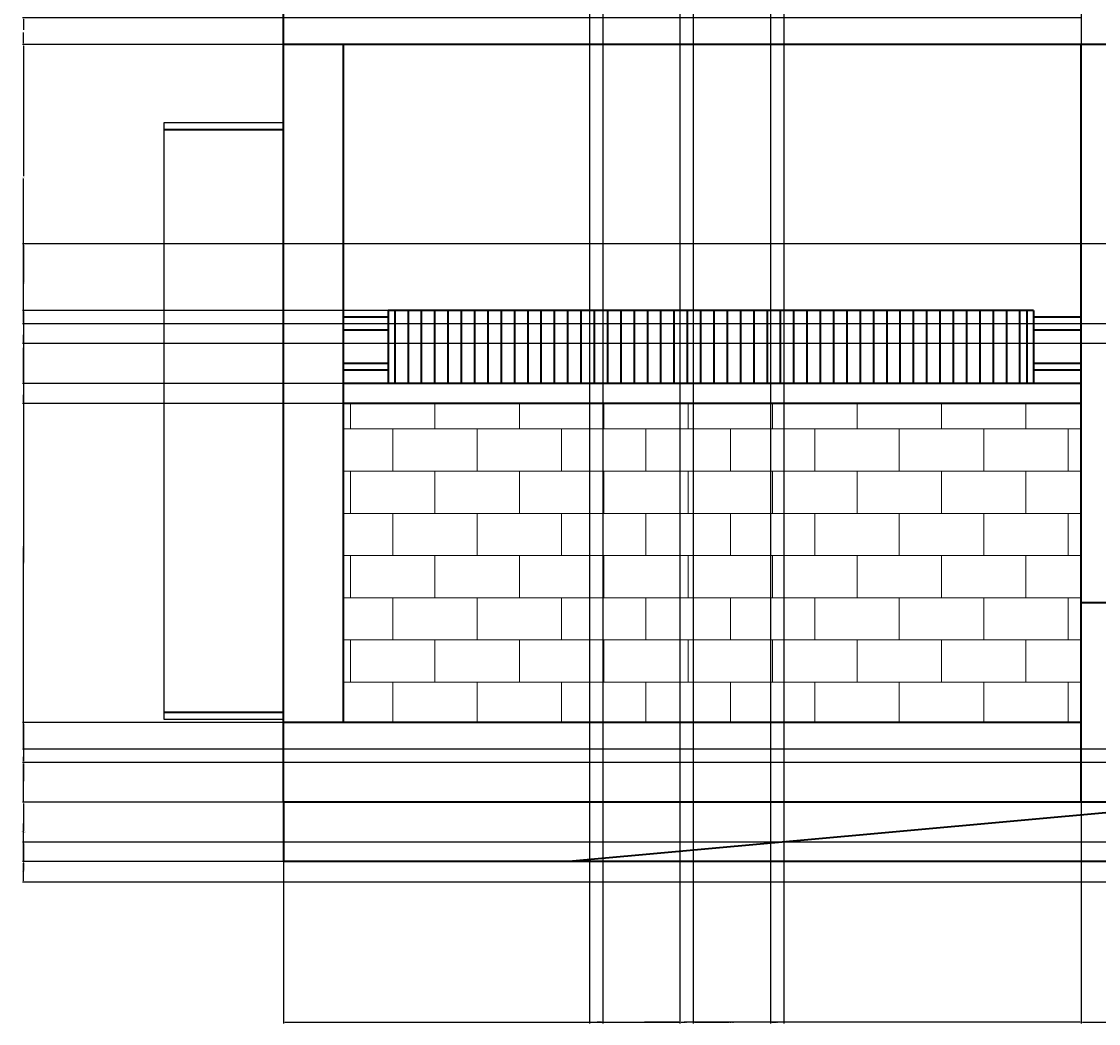
# Model space of a CAD drawing. Units: inches. Extents: x 2148 to 2587, y 1015 to 1466.
# Tile 1 of 7: x 2148 to 2310, y 1015 to 1166. Entities that reach past the tile are written whole.
import ezdxf

# ---------------------------------------------------------------- set-up
doc = ezdxf.new("R2010")
doc.units = ezdxf.units.IN
for name, color, linetype, lineweight in [('A-ANNO-DIMS', 2, 'Continuous', 18), ('A-ELEV', 7, 'Continuous', 35), ('A-GLAZ', 4, 'Continuous', 25), ('A-WALL-PATT', 8, 'Continuous', 18)]:
    doc.layers.add(name, color=color, linetype=linetype, lineweight=lineweight)
doc.styles.get("Standard").update_dxf_attribs({"font": 'arial.ttf'})
doc.dimstyles.get("Standard").update_dxf_attribs({"dimtxt": 0.18, "dimasz": 0.18, "dimexe": 0.18, "dimexo": 0.0625, "dimgap": 0.09, "dimtad": 0, "dimtih": 1, "dimtoh": 1, "dimdec": 4, "dimzin": 0, "dimdsep": 46, "dimtxsty": 'Standard', "dimcen": 0.09, "dimadec": 0, "dimazin": 0, "dimtfac": 1, "dimtdec": 4, "dimtofl": 0, "dimtmove": 0, "dimatfit": 3, "dimfxl": 1, "dimtolj": 1, "dimtzin": 0, "dimarcsym": 0})

# ---------------------------------------------------------------- blocks, each defined once
blk = doc.blocks.new('WIN-SIDE')
for p, q in [((18, 89.73), (0, 89.73)), ((18, 0), (18, 89.73)), ((0, 0), (18, 0))]:
    blk.add_line(p, q)
blk = doc.blocks.new('*D10')
at = {"layer": 'A-ANNO-DIMS', "color": 0, "lineweight": -2, "transparency": 16777216}
for p, q in [((2307.03, 1048.68), (2307.03, 1015.46)), ((2187.03, 1039.75), (2187.03, 1015.46)), ((2187.21, 1015.64), (2246.75, 1015.64)), ((2306.85, 1015.64), (2247.31, 1015.64))]:
    blk.add_line(p, q, dxfattribs=at)
at = {"layer": 'A-ANNO-DIMS', "color": 0, "transparency": 16777216}
for points in [[(2187.21, 1015.67), (2187.21, 1015.61), (2187.03, 1015.64)], [(2306.85, 1015.67), (2306.85, 1015.61), (2307.03, 1015.64)]]:
    blk.add_solid(points, dxfattribs=at)
at = {"layer": 'Defpoints', "color": 0, "transparency": 16777216}
for p in [(2307.03, 1048.74), (2187.03, 1039.82), (2307.03, 1015.64)]:
    blk.add_point(p, dxfattribs=at)
at = {"layer": 'A-ANNO-DIMS', "color": 0, "transparency": 16777216, "insert": (2247.03, 1015.64), "char_height": 0.18, "attachment_point": 5}
blk.add_mtext('\\A1;120', dxfattribs=at)
blk = doc.blocks.new('*D11')
at = {"layer": 'A-ANNO-DIMS', "color": 0, "lineweight": -2, "transparency": 16777216}
for p, q in [((2307.03, 1048.68), (2307.03, 1015.46)), ((2316.03, 1048.68), (2316.03, 1015.46)), ((2307.21, 1015.64), (2311.39, 1015.64)), ((2315.85, 1015.64), (2311.68, 1015.64))]:
    blk.add_line(p, q, dxfattribs=at)
at = {"layer": 'A-ANNO-DIMS', "color": 0, "transparency": 16777216}
for points in [[(2307.21, 1015.67), (2307.21, 1015.61), (2307.03, 1015.64)], [(2315.85, 1015.67), (2315.85, 1015.61), (2316.03, 1015.64)]]:
    blk.add_solid(points, dxfattribs=at)
at = {"layer": 'Defpoints', "color": 0, "transparency": 16777216}
for p in [(2307.03, 1048.74), (2316.03, 1048.74), (2316.03, 1015.64)]:
    blk.add_point(p, dxfattribs=at)
at = {"layer": 'A-ANNO-DIMS', "color": 0, "transparency": 16777216, "insert": (2311.53, 1015.64), "char_height": 0.18, "attachment_point": 5}
blk.add_mtext('\\A1;9', dxfattribs=at)
blk = doc.blocks.new('*D16')
at = {"layer": 'A-ANNO-DIMS', "color": 0, "lineweight": -2, "transparency": 16777216}
for p, q in [((2186.97, 1048.74), (2147.75, 1048.74)), ((2147.93, 1048.56), (2147.93, 1044.46)), ((2147.93, 1040), (2147.93, 1044.1)), ((2186.97, 1039.82), (2147.75, 1039.82))]:
    blk.add_line(p, q, dxfattribs=at)
at = {"layer": 'A-ANNO-DIMS', "color": 0, "transparency": 16777216}
for points in [[(2147.9, 1048.56), (2147.96, 1048.56), (2147.93, 1048.74)], [(2147.9, 1040), (2147.96, 1040), (2147.93, 1039.82)]]:
    blk.add_solid(points, dxfattribs=at)
at = {"layer": 'Defpoints', "color": 0, "transparency": 16777216}
for p in [(2147.93, 1048.74), (2187.03, 1048.74), (2187.03, 1039.82)]:
    blk.add_point(p, dxfattribs=at)
at = {"layer": 'A-ANNO-DIMS', "color": 0, "transparency": 16777216, "insert": (2147.93, 1044.28), "char_height": 0.18, "attachment_point": 5}
blk.add_mtext('\\A1;8.925', dxfattribs=at)
blk = doc.blocks.new('*D17')
at = {"layer": 'A-ANNO-DIMS', "color": 0, "lineweight": -2, "transparency": 16777216}
for p, q in [((2186.97, 1060.74), (2147.75, 1060.74)), ((2147.93, 1060.56), (2147.93, 1054.92)), ((2147.93, 1048.92), (2147.93, 1054.56)), ((2186.97, 1048.74), (2147.75, 1048.74))]:
    blk.add_line(p, q, dxfattribs=at)
at = {"layer": 'A-ANNO-DIMS', "color": 0, "transparency": 16777216}
for points in [[(2147.9, 1060.56), (2147.96, 1060.56), (2147.93, 1060.74)], [(2147.9, 1048.92), (2147.96, 1048.92), (2147.93, 1048.74)]]:
    blk.add_solid(points, dxfattribs=at)
at = {"layer": 'Defpoints', "color": 0, "transparency": 16777216}
for p in [(2147.93, 1060.74), (2187.03, 1060.74), (2187.03, 1048.74)]:
    blk.add_point(p, dxfattribs=at)
at = {"layer": 'A-ANNO-DIMS', "color": 0, "transparency": 16777216, "insert": (2147.93, 1054.74), "char_height": 0.18, "attachment_point": 5}
blk.add_mtext('\\A1;12', dxfattribs=at)
blk = doc.blocks.new('*D18')
at = {"layer": 'A-ANNO-DIMS', "color": 0, "lineweight": -2, "transparency": 16777216}
for p, q in [((2195.97, 1108.74), (2147.75, 1108.74)), ((2147.93, 1108.56), (2147.93, 1084.92)), ((2147.93, 1060.92), (2147.93, 1084.56)), ((2195.97, 1060.74), (2147.75, 1060.74))]:
    blk.add_line(p, q, dxfattribs=at)
at = {"layer": 'A-ANNO-DIMS', "color": 0, "transparency": 16777216}
for points in [[(2147.9, 1108.56), (2147.96, 1108.56), (2147.93, 1108.74)], [(2147.9, 1060.92), (2147.96, 1060.92), (2147.93, 1060.74)]]:
    blk.add_solid(points, dxfattribs=at)
at = {"layer": 'Defpoints', "color": 0, "transparency": 16777216}
for p in [(2147.93, 1108.74), (2196.03, 1108.74), (2196.03, 1060.74)]:
    blk.add_point(p, dxfattribs=at)
at = {"layer": 'A-ANNO-DIMS', "color": 0, "transparency": 16777216, "insert": (2147.93, 1084.74), "char_height": 0.18, "attachment_point": 5}
blk.add_mtext('\\A1;48', dxfattribs=at)
blk = doc.blocks.new('*D19')
at = {"layer": 'A-ANNO-DIMS', "color": 0, "lineweight": -2, "transparency": 16777216}
for p, q in [((2195.97, 1111.74), (2147.75, 1111.74)), ((2147.93, 1111.56), (2147.93, 1110.42)), ((2147.93, 1108.92), (2147.93, 1110.06)), ((2195.97, 1108.74), (2147.75, 1108.74))]:
    blk.add_line(p, q, dxfattribs=at)
at = {"layer": 'A-ANNO-DIMS', "color": 0, "transparency": 16777216}
for points in [[(2147.9, 1111.56), (2147.96, 1111.56), (2147.93, 1111.74)], [(2147.9, 1108.92), (2147.96, 1108.92), (2147.93, 1108.74)]]:
    blk.add_solid(points, dxfattribs=at)
at = {"layer": 'Defpoints', "color": 0, "transparency": 16777216}
for p in [(2147.93, 1111.74), (2196.03, 1111.74), (2196.03, 1108.74)]:
    blk.add_point(p, dxfattribs=at)
at = {"layer": 'A-ANNO-DIMS', "color": 0, "transparency": 16777216, "insert": (2147.93, 1110.24), "char_height": 0.18, "attachment_point": 5}
blk.add_mtext('\\A1;3', dxfattribs=at)
blk = doc.blocks.new('*D20')
at = {"layer": 'A-ANNO-DIMS', "color": 0, "lineweight": -2, "transparency": 16777216}
for p, q in [((2202.7, 1122.74), (2147.75, 1122.74)), ((2147.93, 1122.56), (2147.93, 1117.42)), ((2147.93, 1111.92), (2147.93, 1117.06)), ((2202.7, 1111.74), (2147.75, 1111.74))]:
    blk.add_line(p, q, dxfattribs=at)
at = {"layer": 'A-ANNO-DIMS', "color": 0, "transparency": 16777216}
for points in [[(2147.9, 1122.56), (2147.96, 1122.56), (2147.93, 1122.74)], [(2147.9, 1111.92), (2147.96, 1111.92), (2147.93, 1111.74)]]:
    blk.add_solid(points, dxfattribs=at)
at = {"layer": 'Defpoints', "color": 0, "transparency": 16777216}
for p in [(2147.93, 1122.74), (2202.76, 1122.74), (2202.76, 1111.74)]:
    blk.add_point(p, dxfattribs=at)
at = {"layer": 'A-ANNO-DIMS', "color": 0, "transparency": 16777216, "insert": (2147.93, 1117.24), "char_height": 0.18, "attachment_point": 5}
blk.add_mtext('\\A1;11', dxfattribs=at)
blk = doc.blocks.new('*D21')
at = {"layer": 'A-ANNO-DIMS', "color": 0, "lineweight": -2, "transparency": 16777216}
for p, q in [((2186.97, 1162.74), (2147.75, 1162.74)), ((2147.93, 1162.56), (2147.93, 1142.92)), ((2147.93, 1122.92), (2147.93, 1142.56)), ((2202.7, 1122.74), (2147.75, 1122.74))]:
    blk.add_line(p, q, dxfattribs=at)
at = {"layer": 'A-ANNO-DIMS', "color": 0, "transparency": 16777216}
for points in [[(2147.9, 1162.56), (2147.96, 1162.56), (2147.93, 1162.74)], [(2147.9, 1122.92), (2147.96, 1122.92), (2147.93, 1122.74)]]:
    blk.add_solid(points, dxfattribs=at)
at = {"layer": 'Defpoints', "color": 0, "transparency": 16777216}
for p in [(2147.93, 1162.74), (2187.03, 1162.74), (2202.76, 1122.74)]:
    blk.add_point(p, dxfattribs=at)
at = {"layer": 'A-ANNO-DIMS', "color": 0, "transparency": 16777216, "insert": (2147.93, 1142.74), "char_height": 0.18, "attachment_point": 5}
blk.add_mtext('\\A1;40', dxfattribs=at)
blk = doc.blocks.new('*D22')
at = {"layer": 'A-ANNO-DIMS', "color": 0, "lineweight": -2, "transparency": 16777216}
for p, q in [((2186.971769, 1166.74266), (2147.754269, 1166.74266)), ((2147.934269, 1166.56266), (2147.934269, 1164.92266)), ((2147.934269, 1162.92266), (2147.934269, 1164.56266)), ((2186.971769, 1162.74266), (2147.754269, 1162.74266))]:
    blk.add_line(p, q, dxfattribs=at)
at = {"layer": 'A-ANNO-DIMS', "color": 0, "transparency": 16777216}
for points in [[(2147.904269, 1166.56266), (2147.964269, 1166.56266), (2147.934269, 1166.74266)], [(2147.904269, 1162.92266), (2147.964269, 1162.92266), (2147.934269, 1162.74266)]]:
    blk.add_solid(points, dxfattribs=at)
at = {"layer": 'Defpoints', "color": 0, "transparency": 16777216}
for p in [(2147.934269, 1166.74266), (2187.034269, 1166.74266), (2187.034269, 1162.74266)]:
    blk.add_point(p, dxfattribs=at)
at = {"layer": 'A-ANNO-DIMS', "color": 0, "transparency": 16777216, "insert": (2147.934269, 1164.74266), "char_height": 0.18, "attachment_point": 5}
blk.add_mtext('\\A1;4', dxfattribs=at)
blk = doc.blocks.new('*D47')
at = {"layer": 'A-ANNO-DIMS', "color": 0, "lineweight": -2, "transparency": 16777216}
for p, q in [((2307.03, 1334.68), (2307.03, 1015.46)), ((2316.03, 1329.68), (2316.03, 1015.46)), ((2307.21, 1015.64), (2311.39, 1015.64)), ((2315.85, 1015.64), (2311.68, 1015.64))]:
    blk.add_line(p, q, dxfattribs=at)
at = {"layer": 'A-ANNO-DIMS', "color": 0, "transparency": 16777216}
for points in [[(2307.21, 1015.67), (2307.21, 1015.61), (2307.03, 1015.64)], [(2315.85, 1015.67), (2315.85, 1015.61), (2316.03, 1015.64)]]:
    blk.add_solid(points, dxfattribs=at)
at = {"layer": 'Defpoints', "color": 0, "transparency": 16777216}
for p in [(2307.03, 1334.74), (2316.03, 1329.74), (2316.03, 1015.64)]:
    blk.add_point(p, dxfattribs=at)
at = {"layer": 'A-ANNO-DIMS', "color": 0, "transparency": 16777216, "insert": (2311.53, 1015.64), "char_height": 0.18, "attachment_point": 5}
blk.add_mtext('\\A1;9', dxfattribs=at)
blk = doc.blocks.new('*D58')
at = {"layer": 'A-ANNO-DIMS', "color": 0, "lineweight": -2, "transparency": 16777216}
for p, q in [((2306.971769, 1166.74266), (2147.754269, 1166.74266)), ((2147.934269, 1166.56266), (2147.934269, 1164.92266)), ((2147.934269, 1162.92266), (2147.934269, 1164.56266)), ((2306.971769, 1162.74266), (2147.754269, 1162.74266))]:
    blk.add_line(p, q, dxfattribs=at)
at = {"layer": 'A-ANNO-DIMS', "color": 0, "transparency": 16777216}
for points in [[(2147.904269, 1166.56266), (2147.964269, 1166.56266), (2147.934269, 1166.74266)], [(2147.904269, 1162.92266), (2147.964269, 1162.92266), (2147.934269, 1162.74266)]]:
    blk.add_solid(points, dxfattribs=at)
at = {"layer": 'Defpoints', "color": 0, "transparency": 16777216}
for p in [(2147.934269, 1166.74266), (2307.034269, 1166.74266), (2307.034269, 1162.74266)]:
    blk.add_point(p, dxfattribs=at)
at = {"layer": 'A-ANNO-DIMS', "color": 0, "transparency": 16777216, "insert": (2147.934269, 1164.74266), "char_height": 0.18, "attachment_point": 5}
blk.add_mtext('\\A1;4', dxfattribs=at)
blk = doc.blocks.new('*D83')
at = {"layer": 'A-ANNO-DIMS', "color": 0, "lineweight": -2, "transparency": 16777216}
for p, q in [((2235.06, 1199.68), (2235.06, 1015.46)), ((2233.06, 1197.68), (2233.06, 1015.46)), ((2233.24, 1015.64), (2233.91, 1015.64)), ((2234.88, 1015.64), (2234.21, 1015.64))]:
    blk.add_line(p, q, dxfattribs=at)
at = {"layer": 'A-ANNO-DIMS', "color": 0, "transparency": 16777216}
for points in [[(2233.24, 1015.67), (2233.24, 1015.61), (2233.06, 1015.64)], [(2234.88, 1015.67), (2234.88, 1015.61), (2235.06, 1015.64)]]:
    blk.add_solid(points, dxfattribs=at)
at = {"layer": 'Defpoints', "color": 0, "transparency": 16777216}
for p in [(2235.06, 1199.74), (2233.06, 1197.74), (2235.06, 1015.64)]:
    blk.add_point(p, dxfattribs=at)
at = {"layer": 'A-ANNO-DIMS', "color": 0, "transparency": 16777216, "insert": (2234.06, 1015.64), "char_height": 0.18, "attachment_point": 5}
blk.add_mtext('\\A1;2', dxfattribs=at)
blk = doc.blocks.new('*D84')
at = {"layer": 'A-ANNO-DIMS', "color": 0, "lineweight": -2, "transparency": 16777216}
for p, q in [((2246.67, 1247.43), (2246.67, 1015.46)), ((2235.06, 1199.68), (2235.06, 1015.46)), ((2235.24, 1015.64), (2240.41, 1015.64)), ((2246.49, 1015.64), (2241.32, 1015.64))]:
    blk.add_line(p, q, dxfattribs=at)
at = {"layer": 'A-ANNO-DIMS', "color": 0, "transparency": 16777216}
for points in [[(2235.24, 1015.67), (2235.24, 1015.61), (2235.06, 1015.64)], [(2246.49, 1015.67), (2246.49, 1015.61), (2246.67, 1015.64)]]:
    blk.add_solid(points, dxfattribs=at)
at = {"layer": 'Defpoints', "color": 0, "transparency": 16777216}
for p in [(2246.67, 1247.49), (2235.06, 1199.74), (2246.67, 1015.64)]:
    blk.add_point(p, dxfattribs=at)
at = {"layer": 'A-ANNO-DIMS', "color": 0, "transparency": 16777216, "insert": (2240.87, 1015.64), "char_height": 0.18, "attachment_point": 5}
blk.add_mtext('\\A1;11.613', dxfattribs=at)
blk = doc.blocks.new('*D85')
at = {"layer": 'A-ANNO-DIMS', "color": 0, "lineweight": -2, "transparency": 16777216}
for p, q in [((2246.67, 1247.43), (2246.67, 1015.46)), ((2248.67, 1247.43), (2248.67, 1015.46)), ((2246.85, 1015.64), (2247.52, 1015.64)), ((2248.49, 1015.64), (2247.82, 1015.64))]:
    blk.add_line(p, q, dxfattribs=at)
at = {"layer": 'A-ANNO-DIMS', "color": 0, "transparency": 16777216}
for points in [[(2246.85, 1015.67), (2246.85, 1015.61), (2246.67, 1015.64)], [(2248.49, 1015.67), (2248.49, 1015.61), (2248.67, 1015.64)]]:
    blk.add_solid(points, dxfattribs=at)
at = {"layer": 'Defpoints', "color": 0, "transparency": 16777216}
for p in [(2246.67, 1247.49), (2248.67, 1247.49), (2248.67, 1015.64)]:
    blk.add_point(p, dxfattribs=at)
at = {"layer": 'A-ANNO-DIMS', "color": 0, "transparency": 16777216, "insert": (2247.67, 1015.64), "char_height": 0.18, "attachment_point": 5}
blk.add_mtext('\\A1;2', dxfattribs=at)
blk = doc.blocks.new('*D86')
at = {"layer": 'A-ANNO-DIMS', "color": 0, "lineweight": -2, "transparency": 16777216}
for p, q in [((2248.67, 1247.43), (2248.67, 1015.46)), ((2260.29, 1199.68), (2260.29, 1015.46)), ((2248.85, 1015.64), (2254.03, 1015.64)), ((2260.11, 1015.64), (2254.94, 1015.64))]:
    blk.add_line(p, q, dxfattribs=at)
at = {"layer": 'A-ANNO-DIMS', "color": 0, "transparency": 16777216}
for points in [[(2248.85, 1015.67), (2248.85, 1015.61), (2248.67, 1015.64)], [(2260.11, 1015.67), (2260.11, 1015.61), (2260.29, 1015.64)]]:
    blk.add_solid(points, dxfattribs=at)
at = {"layer": 'Defpoints', "color": 0, "transparency": 16777216}
for p in [(2248.67, 1247.49), (2260.29, 1199.74), (2260.29, 1015.64)]:
    blk.add_point(p, dxfattribs=at)
at = {"layer": 'A-ANNO-DIMS', "color": 0, "transparency": 16777216, "insert": (2254.48, 1015.64), "char_height": 0.18, "attachment_point": 5}
blk.add_mtext('\\A1;11.613', dxfattribs=at)
blk = doc.blocks.new('*D87')
at = {"layer": 'A-ANNO-DIMS', "color": 0, "lineweight": -2, "transparency": 16777216}
for p, q in [((2260.29, 1199.68), (2260.29, 1015.46)), ((2262.29, 1197.68), (2262.29, 1015.46)), ((2260.47, 1015.64), (2261.14, 1015.64)), ((2262.11, 1015.64), (2261.44, 1015.64))]:
    blk.add_line(p, q, dxfattribs=at)
at = {"layer": 'A-ANNO-DIMS', "color": 0, "transparency": 16777216}
for points in [[(2260.47, 1015.67), (2260.47, 1015.61), (2260.29, 1015.64)], [(2262.11, 1015.67), (2262.11, 1015.61), (2262.29, 1015.64)]]:
    blk.add_solid(points, dxfattribs=at)
at = {"layer": 'Defpoints', "color": 0, "transparency": 16777216}
for p in [(2260.29, 1199.74), (2262.29, 1197.74), (2262.29, 1015.64)]:
    blk.add_point(p, dxfattribs=at)
at = {"layer": 'A-ANNO-DIMS', "color": 0, "transparency": 16777216, "insert": (2261.29, 1015.64), "char_height": 0.18, "attachment_point": 5}
blk.add_mtext('\\A1;2', dxfattribs=at)
blk = doc.blocks.new('*D110')
at = {"layer": 'A-ANNO-DIMS', "color": 0, "lineweight": -2, "transparency": 16777216}
for p, q in [((2327.97, 1039.82), (2147.75, 1039.82)), ((2147.93, 1039.64), (2147.93, 1038.46)), ((2327.97, 1036.74), (2147.75, 1036.74)), ((2147.93, 1036.92), (2147.93, 1038.1))]:
    blk.add_line(p, q, dxfattribs=at)
at = {"layer": 'A-ANNO-DIMS', "color": 0, "transparency": 16777216}
for points in [[(2147.9, 1039.64), (2147.96, 1039.64), (2147.93, 1039.82)], [(2147.9, 1036.92), (2147.96, 1036.92), (2147.93, 1036.74)]]:
    blk.add_solid(points, dxfattribs=at)
at = {"layer": 'Defpoints', "color": 0, "transparency": 16777216}
for p in [(2147.93, 1039.82), (2328.03, 1039.82), (2328.03, 1036.74)]:
    blk.add_point(p, dxfattribs=at)
at = {"layer": 'A-ANNO-DIMS', "color": 0, "transparency": 16777216, "insert": (2147.93, 1038.28), "char_height": 0.18, "attachment_point": 5}
blk.add_mtext('\\A1;3.07', dxfattribs=at)
blk = doc.blocks.new('*D111')
at = {"layer": 'A-ANNO-DIMS', "color": 0, "lineweight": -2, "transparency": 16777216}
for p, q in [((2327.97, 1048.74), (2147.75, 1048.74)), ((2147.93, 1048.56), (2147.93, 1044.46)), ((2147.93, 1040), (2147.93, 1044.1)), ((2327.97, 1039.82), (2147.75, 1039.82))]:
    blk.add_line(p, q, dxfattribs=at)
at = {"layer": 'A-ANNO-DIMS', "color": 0, "transparency": 16777216}
for points in [[(2147.9, 1048.56), (2147.96, 1048.56), (2147.93, 1048.74)], [(2147.9, 1040), (2147.96, 1040), (2147.93, 1039.82)]]:
    blk.add_solid(points, dxfattribs=at)
at = {"layer": 'Defpoints', "color": 0, "transparency": 16777216}
for p in [(2147.93, 1048.74), (2328.03, 1048.74), (2328.03, 1039.82)]:
    blk.add_point(p, dxfattribs=at)
at = {"layer": 'A-ANNO-DIMS', "color": 0, "transparency": 16777216, "insert": (2147.93, 1044.28), "char_height": 0.18, "attachment_point": 5}
blk.add_mtext('\\A1;8.925', dxfattribs=at)
blk = doc.blocks.new('*D112')
at = {"layer": 'A-ANNO-DIMS', "color": 0, "lineweight": -2, "transparency": 16777216}
for p, q in [((2327.97, 1054.74), (2147.75, 1054.74)), ((2147.93, 1054.56), (2147.93, 1051.92)), ((2147.93, 1048.92), (2147.93, 1051.56)), ((2327.97, 1048.74), (2147.75, 1048.74))]:
    blk.add_line(p, q, dxfattribs=at)
at = {"layer": 'A-ANNO-DIMS', "color": 0, "transparency": 16777216}
for points in [[(2147.9, 1054.56), (2147.96, 1054.56), (2147.93, 1054.74)], [(2147.9, 1048.92), (2147.96, 1048.92), (2147.93, 1048.74)]]:
    blk.add_solid(points, dxfattribs=at)
at = {"layer": 'Defpoints', "color": 0, "transparency": 16777216}
for p in [(2147.93, 1054.74), (2328.03, 1054.74), (2328.03, 1048.74)]:
    blk.add_point(p, dxfattribs=at)
at = {"layer": 'A-ANNO-DIMS', "color": 0, "transparency": 16777216, "insert": (2147.93, 1051.74), "char_height": 0.18, "attachment_point": 5}
blk.add_mtext('\\A1;6', dxfattribs=at)
blk = doc.blocks.new('*D113')
at = {"layer": 'A-ANNO-DIMS', "color": 0, "lineweight": -2, "transparency": 16777216}
for p, q in [((2334.97, 1056.74), (2147.75, 1056.74)), ((2147.93, 1056.56), (2147.93, 1055.92)), ((2327.97, 1054.74), (2147.75, 1054.74)), ((2147.93, 1054.92), (2147.93, 1055.56))]:
    blk.add_line(p, q, dxfattribs=at)
at = {"layer": 'A-ANNO-DIMS', "color": 0, "transparency": 16777216}
for points in [[(2147.9, 1056.56), (2147.96, 1056.56), (2147.93, 1056.74)], [(2147.9, 1054.92), (2147.96, 1054.92), (2147.93, 1054.74)]]:
    blk.add_solid(points, dxfattribs=at)
at = {"layer": 'Defpoints', "color": 0, "transparency": 16777216}
for p in [(2147.93, 1056.74), (2335.03, 1056.74), (2328.03, 1054.74)]:
    blk.add_point(p, dxfattribs=at)
at = {"layer": 'A-ANNO-DIMS', "color": 0, "transparency": 16777216, "insert": (2147.93, 1055.74), "char_height": 0.18, "attachment_point": 5}
blk.add_mtext('\\A1;2', dxfattribs=at)
blk = doc.blocks.new('*D114')
at = {"layer": 'A-ANNO-DIMS', "color": 0, "lineweight": -2, "transparency": 16777216}
for p, q in [((2330.97, 1117.74), (2147.75, 1117.74)), ((2147.93, 1117.56), (2147.93, 1087.42)), ((2147.93, 1056.92), (2147.93, 1087.06)), ((2334.97, 1056.74), (2147.75, 1056.74))]:
    blk.add_line(p, q, dxfattribs=at)
at = {"layer": 'A-ANNO-DIMS', "color": 0, "transparency": 16777216}
for points in [[(2147.9, 1117.56), (2147.96, 1117.56), (2147.93, 1117.74)], [(2147.9, 1056.92), (2147.96, 1056.92), (2147.93, 1056.74)]]:
    blk.add_solid(points, dxfattribs=at)
at = {"layer": 'Defpoints', "color": 0, "transparency": 16777216}
for p in [(2147.93, 1117.74), (2331.03, 1117.74), (2335.03, 1056.74)]:
    blk.add_point(p, dxfattribs=at)
at = {"layer": 'A-ANNO-DIMS', "color": 0, "transparency": 16777216, "insert": (2147.93, 1087.24), "char_height": 0.18, "attachment_point": 5}
blk.add_mtext('\\A1;61', dxfattribs=at)
blk = doc.blocks.new('*D115')
at = {"layer": 'A-ANNO-DIMS', "color": 0, "lineweight": -2, "transparency": 16777216}
for p, q in [((2327.97, 1120.74), (2147.75, 1120.74)), ((2147.93, 1120.56), (2147.93, 1119.42)), ((2330.97, 1117.74), (2147.75, 1117.74)), ((2147.93, 1117.92), (2147.93, 1119.06))]:
    blk.add_line(p, q, dxfattribs=at)
at = {"layer": 'A-ANNO-DIMS', "color": 0, "transparency": 16777216}
for points in [[(2147.9, 1120.56), (2147.96, 1120.56), (2147.93, 1120.74)], [(2147.9, 1117.92), (2147.96, 1117.92), (2147.93, 1117.74)]]:
    blk.add_solid(points, dxfattribs=at)
at = {"layer": 'Defpoints', "color": 0, "transparency": 16777216}
for p in [(2147.93, 1120.74), (2328.03, 1120.74), (2331.03, 1117.74)]:
    blk.add_point(p, dxfattribs=at)
at = {"layer": 'A-ANNO-DIMS', "color": 0, "transparency": 16777216, "insert": (2147.93, 1119.24), "char_height": 0.18, "attachment_point": 5}
blk.add_mtext('\\A1;3', dxfattribs=at)
blk = doc.blocks.new('*D116')
at = {"layer": 'A-ANNO-DIMS', "color": 0, "lineweight": -2, "transparency": 16777216}
for p, q in [((2327.97, 1132.74), (2147.75, 1132.74)), ((2147.93, 1132.56), (2147.93, 1126.92)), ((2147.93, 1120.92), (2147.93, 1126.56)), ((2327.97, 1120.74), (2147.75, 1120.74))]:
    blk.add_line(p, q, dxfattribs=at)
at = {"layer": 'A-ANNO-DIMS', "color": 0, "transparency": 16777216}
for points in [[(2147.9, 1132.56), (2147.96, 1132.56), (2147.93, 1132.74)], [(2147.9, 1120.92), (2147.96, 1120.92), (2147.93, 1120.74)]]:
    blk.add_solid(points, dxfattribs=at)
at = {"layer": 'Defpoints', "color": 0, "transparency": 16777216}
for p in [(2147.93, 1132.74), (2328.03, 1132.74), (2328.03, 1120.74)]:
    blk.add_point(p, dxfattribs=at)
at = {"layer": 'A-ANNO-DIMS', "color": 0, "transparency": 16777216, "insert": (2147.93, 1126.74), "char_height": 0.18, "attachment_point": 5}
blk.add_mtext('\\A1;12', dxfattribs=at)
blk = doc.blocks.new('*D117')
at = {"layer": 'A-ANNO-DIMS', "color": 0, "lineweight": -2, "transparency": 16777216}
for p, q in [((2403.32, 1042.74), (2147.75, 1042.74)), ((2147.93, 1042.56), (2147.93, 1039.92)), ((2147.93, 1036.92), (2147.93, 1039.56)), ((2404.63, 1036.74), (2147.75, 1036.74))]:
    blk.add_line(p, q, dxfattribs=at)
at = {"layer": 'A-ANNO-DIMS', "color": 0, "transparency": 16777216}
for points in [[(2147.9, 1042.56), (2147.96, 1042.56), (2147.93, 1042.74)], [(2147.9, 1036.92), (2147.96, 1036.92), (2147.93, 1036.74)]]:
    blk.add_solid(points, dxfattribs=at)
at = {"layer": 'Defpoints', "color": 0, "transparency": 16777216}
for p in [(2147.93, 1042.74), (2403.39, 1042.74), (2404.7, 1036.74)]:
    blk.add_point(p, dxfattribs=at)
at = {"layer": 'A-ANNO-DIMS', "color": 0, "transparency": 16777216, "insert": (2147.93, 1039.74), "char_height": 0.18, "attachment_point": 5}
blk.add_mtext('\\A1;6', dxfattribs=at)
blk = doc.blocks.new('*D118')
at = {"layer": 'A-ANNO-DIMS', "color": 0, "lineweight": -2, "transparency": 16777216}
for p, q in [((2402.02, 1048.74), (2147.75, 1048.74)), ((2147.93, 1048.56), (2147.93, 1045.92)), ((2147.93, 1042.92), (2147.93, 1045.56)), ((2403.32, 1042.74), (2147.75, 1042.74))]:
    blk.add_line(p, q, dxfattribs=at)
at = {"layer": 'A-ANNO-DIMS', "color": 0, "transparency": 16777216}
for points in [[(2147.9, 1048.56), (2147.96, 1048.56), (2147.93, 1048.74)], [(2147.9, 1042.92), (2147.96, 1042.92), (2147.93, 1042.74)]]:
    blk.add_solid(points, dxfattribs=at)
at = {"layer": 'Defpoints', "color": 0, "transparency": 16777216}
for p in [(2147.93, 1048.74), (2402.08, 1048.74), (2403.39, 1042.74)]:
    blk.add_point(p, dxfattribs=at)
at = {"layer": 'A-ANNO-DIMS', "color": 0, "transparency": 16777216, "insert": (2147.93, 1045.74), "char_height": 0.18, "attachment_point": 5}
blk.add_mtext('\\A1;6', dxfattribs=at)
blk = doc.blocks.new('*D119')
at = {"layer": 'A-ANNO-DIMS', "color": 0, "lineweight": -2, "transparency": 16777216}
for p, q in [((2400.71, 1054.74), (2147.75, 1054.74)), ((2147.93, 1054.56), (2147.93, 1051.92)), ((2147.93, 1048.92), (2147.93, 1051.56)), ((2402.02, 1048.74), (2147.75, 1048.74))]:
    blk.add_line(p, q, dxfattribs=at)
at = {"layer": 'A-ANNO-DIMS', "color": 0, "transparency": 16777216}
for points in [[(2147.9, 1054.56), (2147.96, 1054.56), (2147.93, 1054.74)], [(2147.9, 1048.92), (2147.96, 1048.92), (2147.93, 1048.74)]]:
    blk.add_solid(points, dxfattribs=at)
at = {"layer": 'Defpoints', "color": 0, "transparency": 16777216}
for p in [(2147.93, 1054.74), (2400.77, 1054.74), (2402.08, 1048.74)]:
    blk.add_point(p, dxfattribs=at)
at = {"layer": 'A-ANNO-DIMS', "color": 0, "transparency": 16777216, "insert": (2147.93, 1051.74), "char_height": 0.18, "attachment_point": 5}
blk.add_mtext('\\A1;6', dxfattribs=at)

msp = doc.modelspace()

# ---------------------------------------------------------------- hatches: boundary and pattern name
at = {"layer": 'A-WALL-PATT'}
h = msp.add_hatch(dxfattribs=at)
h.set_pattern_fill('BRICK', color=256)
h.paths.add_polyline_path([(2307.0343, 1108.7427), (2196.0343, 1108.7427), (2196.0343, 1060.7427), (2307.0343, 1060.7427)])

# ---------------------------------------------------------------- linework, layer by layer
at = {"layer": 'A-ELEV'}
for p, q in [((2187.0343, 1048.7427), (2187.0343, 1438.7427)), ((2547.0343, 1162.7427), (2187.0343, 1162.7427)), ((2196.0343, 1060.7427), (2196.0343, 1162.7427)), ((2307.0343, 1048.7427), (2307.0343, 1162.7427)), ((2169.0343, 1149.9716), (2187.0343, 1149.9716)), ((2299.8475, 1122.7427), (2202.7603, 1122.7427)), ((2202.7603, 1122.7427), (2202.7603, 1111.7427)), ((2203.7603, 1122.7427), (2203.7603, 1111.7427)), ((2205.7603, 1122.7427), (2205.7603, 1111.7427)), ((2207.7603, 1122.7427), (2207.7603, 1111.7427)), ((2209.7603, 1122.7427), (2209.7603, 1111.7427)), ((2211.7603, 1122.7427), (2211.7603, 1111.7427)), ((2213.7603, 1122.7427), (2213.7603, 1111.7427)), ((2215.7603, 1122.7427), (2215.7603, 1111.7427)), ((2217.7603, 1122.7427), (2217.7603, 1111.7427)), ((2219.7603, 1122.7427), (2219.7603, 1111.7427)), ((2221.7603, 1122.7427), (2221.7603, 1111.7427)), ((2223.7603, 1122.7427), (2223.7603, 1111.7427)), ((2225.7603, 1122.7427), (2225.7603, 1111.7427)), ((2227.7603, 1122.7427), (2227.7603, 1111.7427)), ((2229.7603, 1122.7427), (2229.7603, 1111.7427)), ((2231.7603, 1122.7427), (2231.7603, 1111.7427)), ((2233.7603, 1122.7427), (2233.7603, 1111.7427)), ((2235.7603, 1122.7427), (2235.7603, 1111.7427)), ((2237.7603, 1122.7427), (2237.7603, 1111.7427)), ((2239.7603, 1122.7427), (2239.7603, 1111.7427)), ((2241.7603, 1122.7427), (2241.7603, 1111.7427)), ((2243.7603, 1122.7427), (2243.7603, 1111.7427)), ((2245.7603, 1122.7427), (2245.7603, 1111.7427)), ((2247.7603, 1122.7427), (2247.7603, 1111.7427)), ((2249.7603, 1122.7427), (2249.7603, 1111.7427)), ((2251.7603, 1122.7427), (2251.7603, 1111.7427)), ((2253.7603, 1122.7427), (2253.7603, 1111.7427)), ((2255.7603, 1122.7427), (2255.7603, 1111.7427)), ((2257.7603, 1122.7427), (2257.7603, 1111.7427)), ((2259.7603, 1122.7427), (2259.7603, 1111.7427)), ((2261.7603, 1122.7427), (2261.7603, 1111.7427)), ((2263.7603, 1122.7427), (2263.7603, 1111.7427)), ((2265.7603, 1122.7427), (2265.7603, 1111.7427)), ((2267.7603, 1122.7427), (2267.7603, 1111.7427)), ((2269.7603, 1122.7427), (2269.7603, 1111.7427)), ((2271.7603, 1122.7427), (2271.7603, 1111.7427)), ((2273.7603, 1122.7427), (2273.7603, 1111.7427)), ((2275.7603, 1122.7427), (2275.7603, 1111.7427)), ((2277.7603, 1122.7427), (2277.7603, 1111.7427)), ((2279.7603, 1122.7427), (2279.7603, 1111.7427)), ((2281.7603, 1122.7427), (2281.7603, 1111.7427)), ((2283.7603, 1122.7427), (2283.7603, 1111.7427)), ((2285.7603, 1122.7427), (2285.7603, 1111.7427)), ((2287.7603, 1122.7427), (2287.7603, 1111.7427)), ((2289.7603, 1122.7427), (2289.7603, 1111.7427)), ((2291.7603, 1122.7427), (2291.7603, 1111.7427)), ((2293.7603, 1122.7427), (2293.7603, 1111.7427)), ((2295.7603, 1122.7427), (2295.7603, 1111.7427)), ((2297.7603, 1122.7427), (2297.7603, 1111.7427)), ((2298.8475, 1122.7427), (2298.8475, 1111.7427)), ((2299.8475, 1122.7427), (2299.8475, 1111.7427)), ((2202.7603, 1121.7427), (2196.0343, 1121.7427)), ((2307.0343, 1121.7427), (2299.8475, 1121.7427)), ((2202.7603, 1119.7427), (2196.0343, 1119.7427)), ((2307.0343, 1119.7427), (2299.8475, 1119.7427)), ((2202.7603, 1114.7427), (2196.0343, 1114.7427)), ((2307.0343, 1114.7427), (2299.8475, 1114.7427)), ((2202.7603, 1113.7427), (2196.0343, 1113.7427)), ((2307.0343, 1113.7427), (2299.8475, 1113.7427)), ((2307.0343, 1111.7427), (2196.0343, 1111.7427)), ((2307.0343, 1108.7427), (2196.0343, 1108.7427)), ((2316.0343, 1078.7427), (2307.0343, 1078.7427)), ((2187.0343, 1062.2408), (2169.0343, 1062.2408)), ((2307.0343, 1060.7427), (2187.0343, 1060.7427)), ((2328.0343, 1048.7427), (2187.0343, 1048.7427)), ((2187.0343, 1048.7427), (2187.0343, 1039.8173)), ((2328.0343, 1048.7427), (2229.9391, 1039.8173)), ((2328.0343, 1039.8173), (2187.0343, 1039.8173))]:
    msp.add_line(p, q, dxfattribs=at)

# ---------------------------------------------------------------- block references
at = {"layer": 'A-GLAZ', "rotation": 180}
msp.add_blockref('WIN-SIDE', (2187.0345, 1150.9713), dxfattribs=at)

# ---------------------------------------------------------------- dimensions: what is measured, and where the dimension line sits
at = {"layer": 'A-ANNO-DIMS'}
for base, p1, p2, override, picture, middle in [((2316.0343, 1015.6427), (2307.0343, 1334.7427), (2316.0343, 1329.7427), {"dimdec": 0, "dimlfac": 1, "dimrnd": 0, "dimzin": 0, "dimdsep": 46, "dimlunit": 2}, '*D47', (2311.5343, 1015.6427)), ((2246.6736, 1015.6427), (2235.0602, 1199.738), (2246.6736, 1247.4885), {"dimdec": 3, "dimlfac": 1, "dimrnd": 0, "dimzin": 0, "dimdsep": 46, "dimlunit": 2}, '*D84', (2240.8669, 1015.6427)), ((2248.6736, 1015.6427), (2246.6736, 1247.4885), (2248.6736, 1247.4885), {"dimdec": 0, "dimlfac": 1, "dimrnd": 0, "dimzin": 0, "dimdsep": 46, "dimlunit": 2}, '*D85', (2247.6736, 1015.6427)), ((2260.287, 1015.6427), (2248.6736, 1247.4885), (2260.287, 1199.738), {"dimdec": 3, "dimlfac": 1, "dimrnd": 0, "dimzin": 0, "dimdsep": 46, "dimlunit": 2}, '*D86', (2254.4803, 1015.6427)), ((2235.0602, 1015.6427), (2233.0602, 1197.738), (2235.0602, 1199.738), {"dimdec": 0, "dimlfac": 1, "dimrnd": 0, "dimzin": 0, "dimdsep": 46, "dimlunit": 2}, '*D83', (2234.0602, 1015.6427)), ((2262.287, 1015.6427), (2260.287, 1199.738), (2262.287, 1197.738), {"dimdec": 0, "dimlfac": 1, "dimrnd": 0, "dimzin": 0, "dimdsep": 46, "dimlunit": 2}, '*D87', (2261.287, 1015.6427)), ((2307.0343, 1015.6427), (2187.0343, 1039.8173), (2307.0343, 1048.7427), {"dimdec": 0, "dimlfac": 1, "dimrnd": 0, "dimzin": 0, "dimdsep": 46, "dimlunit": 2}, '*D10', (2247.0343, 1015.6427)), ((2316.0343, 1015.6427), (2307.0343, 1048.7427), (2316.0343, 1048.7427), {"dimdec": 0, "dimlfac": 1, "dimrnd": 0, "dimzin": 0, "dimdsep": 46, "dimlunit": 2}, '*D11', (2311.5343, 1015.6427))]:
    dim = msp.add_linear_dim(base=base, p1=p1, p2=p2, dimstyle='Standard', override=override, dxfattribs=at)
    dim.commit()
    dim.dimension.update_dxf_attribs({"geometry": picture, "text_midpoint": middle})
for base, p1, p2, override, picture, middle in [((2147.9343, 1166.7427), (2187.0343, 1162.7427), (2187.0343, 1166.7427), {"dimdec": 0, "dimlfac": 1, "dimrnd": 0, "dimzin": 0, "dimdsep": 46, "dimlunit": 2}, '*D22', (2147.9343, 1164.7427)), ((2147.9343, 1166.7427), (2307.0343, 1162.7427), (2307.0343, 1166.7427), {"dimdec": 0, "dimlfac": 1, "dimrnd": 0, "dimzin": 0, "dimdsep": 46, "dimlunit": 2}, '*D58', (2147.9343, 1164.7427)), ((2147.9343, 1162.7427), (2202.7603, 1122.7427), (2187.0343, 1162.7427), {"dimdec": 0, "dimlfac": 1, "dimrnd": 0, "dimzin": 0, "dimdsep": 46, "dimlunit": 2}, '*D21', (2147.9343, 1142.7427)), ((2147.9343, 1132.7427), (2328.0343, 1120.7427), (2328.0343, 1132.7427), {"dimdec": 0, "dimlfac": 1, "dimrnd": 0, "dimzin": 0, "dimdsep": 46, "dimlunit": 2}, '*D116', (2147.9343, 1126.7427)), ((2147.9343, 1122.7427), (2202.7603, 1111.7427), (2202.7603, 1122.7427), {"dimdec": 0, "dimlfac": 1, "dimrnd": 0, "dimzin": 0, "dimdsep": 46, "dimlunit": 2}, '*D20', (2147.9343, 1117.2427)), ((2147.9343, 1120.7427), (2331.0343, 1117.7427), (2328.0343, 1120.7427), {"dimdec": 0, "dimlfac": 1, "dimrnd": 0, "dimzin": 0, "dimdsep": 46, "dimlunit": 2}, '*D115', (2147.9343, 1119.2427)), ((2147.9343, 1117.7427), (2335.0343, 1056.7427), (2331.0343, 1117.7427), {"dimdec": 0, "dimlfac": 1, "dimrnd": 0, "dimzin": 0, "dimdsep": 46, "dimlunit": 2}, '*D114', (2147.9343, 1087.2427)), ((2147.9343, 1111.7427), (2196.0343, 1108.7427), (2196.0343, 1111.7427), {"dimdec": 0, "dimlfac": 1, "dimrnd": 0, "dimzin": 0, "dimdsep": 46, "dimlunit": 2}, '*D19', (2147.9343, 1110.2427)), ((2147.9343, 1108.7427), (2196.0343, 1060.7427), (2196.0343, 1108.7427), {"dimdec": 0, "dimlfac": 1, "dimrnd": 0, "dimzin": 0, "dimdsep": 46, "dimlunit": 2}, '*D18', (2147.9343, 1084.7427)), ((2147.9343, 1060.7427), (2187.0343, 1048.7427), (2187.0343, 1060.7427), {"dimdec": 0, "dimlfac": 1, "dimrnd": 0, "dimzin": 0, "dimdsep": 46, "dimlunit": 2}, '*D17', (2147.9343, 1054.7427)), ((2147.9343, 1056.7427), (2328.0343, 1054.7427), (2335.0343, 1056.7427), {"dimdec": 0, "dimlfac": 1, "dimrnd": 0, "dimzin": 0, "dimdsep": 46, "dimlunit": 2}, '*D113', (2147.9343, 1055.7427)), ((2147.9343, 1054.7427), (2328.0343, 1048.7427), (2328.0343, 1054.7427), {"dimdec": 0, "dimlfac": 1, "dimrnd": 0, "dimzin": 0, "dimdsep": 46, "dimlunit": 2}, '*D112', (2147.9343, 1051.7427)), ((2147.9343, 1054.7427), (2402.0782, 1048.7427), (2400.7695, 1054.7427), {"dimdec": 0, "dimlfac": 1, "dimrnd": 0, "dimzin": 0, "dimdsep": 46, "dimlunit": 2}, '*D119', (2147.9343, 1051.7427)), ((2147.9343, 1048.7427), (2187.0343, 1039.8173), (2187.0343, 1048.7427), {"dimdec": 3, "dimlfac": 1, "dimrnd": 0, "dimzin": 0, "dimdsep": 46, "dimlunit": 2}, '*D16', (2147.9343, 1044.28)), ((2147.9343, 1048.7427), (2328.0343, 1039.8173), (2328.0343, 1048.7427), {"dimdec": 3, "dimlfac": 1, "dimrnd": 0, "dimzin": 0, "dimdsep": 46, "dimlunit": 2}, '*D111', (2147.9343, 1044.28)), ((2147.9343, 1048.7427), (2403.3868, 1042.7427), (2402.0782, 1048.7427), {"dimdec": 0, "dimlfac": 1, "dimrnd": 0, "dimzin": 0, "dimdsep": 46, "dimlunit": 2}, '*D118', (2147.9343, 1045.7427)), ((2147.9343, 1042.7427), (2404.6955, 1036.7427), (2403.3868, 1042.7427), {"dimdec": 0, "dimlfac": 1, "dimrnd": 0, "dimzin": 0, "dimdsep": 46, "dimlunit": 2}, '*D117', (2147.9343, 1039.7427)), ((2147.9343, 1039.8173), (2328.0343, 1036.7427), (2328.0343, 1039.8173), {"dimdec": 2, "dimlfac": 1, "dimrnd": 0, "dimzin": 0, "dimdsep": 46, "dimlunit": 2}, '*D110', (2147.9343, 1038.28))]:
    dim = msp.add_linear_dim(base=base, p1=p1, p2=p2, angle=90, dimstyle='Standard', override=override, dxfattribs=at)
    dim.commit()
    dim.dimension.update_dxf_attribs({"geometry": picture, "text_midpoint": middle})

doc.saveas('drawing.dxf')
